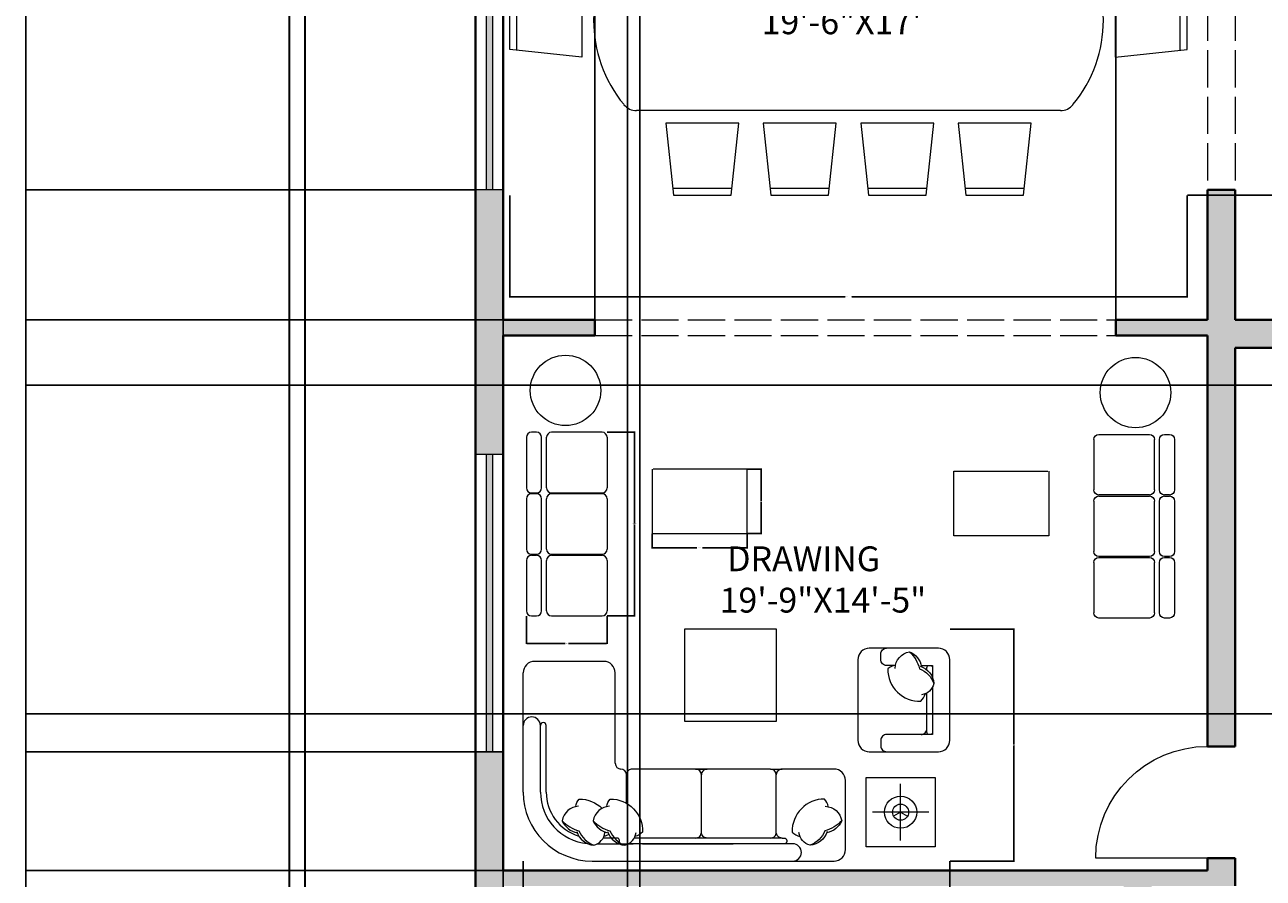
# Model space of a CAD drawing. Units: inches. Extents: x 2330 to 3943, y 1763 to 3461.
# Tile 10 of 40: x 2330 to 2730, y 2554 to 2829. Entities that reach past the tile are written whole.
import ezdxf

# ---------------------------------------------------------------- set-up
doc = ezdxf.new("R2010")
doc.units = ezdxf.units.IN
doc.linetypes.add('ACAD_ISO02W100', pattern=[15, 12, -3])
for name, color, linetype, lineweight in [('A-ANNO-DIMS', 2, 'Continuous', 18), ('A-AREA-IDEN', 7, 'Continuous', 18), ('A-DOOR', 4, 'Continuous', 18), ('A-FURN', 8, 'Continuous', 13), ('A-GLAZ', 4, 'Continuous', 18), ('A-WALL', 7, 'Continuous', 40), ('A-WALL-OVHD', 7, 'ACAD_ISO02W100', 18), ('A-WALL-PATT', 252, 'Continuous', 13), ('C-PROP', 7, 'Continuous', 30)]:
    doc.layers.add(name, color=color, linetype=linetype, lineweight=lineweight)
doc.styles.get("Standard").update_dxf_attribs({"font": 'arial.ttf'})
doc.dimstyles.get("Standard").update_dxf_attribs({"dimtxt": 0.18, "dimasz": 0.18, "dimexe": 0.18, "dimexo": 0.0625, "dimgap": 0.09, "dimtad": 0, "dimtih": 1, "dimtoh": 1, "dimdec": 4, "dimzin": 0, "dimdsep": 46, "dimtxsty": 'Standard', "dimcen": 0.09, "dimadec": 0, "dimazin": 0, "dimtfac": 1, "dimtdec": 4, "dimtofl": 0, "dimtmove": 0, "dimatfit": 3, "dimfxl": 1, "dimtolj": 1, "dimtzin": 0, "dimarcsym": 0})

# ---------------------------------------------------------------- blocks, each defined once
blk = doc.blocks.new('A$C714C64AF')
for p, q in [((3108, 2017, -5499), (1005, 2017, -5499)), ((908, 1917, -5499), (908, 1317, -5499)), ((1365, 1867, -5499), (2793, 1867, -5499)), ((3508, 1417, -5499), (3508, 839, -5499)), ((3558, 1417, -5499), (3558, 839, -5499)), ((3708, 1417, -5499), (3708, 839, -5499)), ((1008, 1217, -5499), (1458, 1217, -5499)), ((1558, 1217, -5499), (1458, 1217, -5499)), ((1558, 1217, -5499), (2760, 1217, -5499)), ((2209, 1217, -5499), (2109, 1217, -5499)), ((2908, 1167, -5499), (2908, 381, -5499)), ((3708, 839, -5499), (3708, 381, -5499)), ((3008, 281, -5499), (3608, 281, -5499))]:
    blk.add_line(p, q)
at = {"elevation": -5499}
for points in [[(128, 1892), (728, 1892), (728, 1292), (128, 1292)], [(2306, 800), (1506, 800), (1506, 0), (2306, 0)]]:
    blk.add_lwpolyline(points, close=True, dxfattribs=at)
for points in [[(428, 1837), (428, 1347)], [(1884, 1867), (2670, 1867)], [(1458, 1817), (2743, 1817)], [(2944, 1817), (3012, 1817)], [(428, 1592), (367, 1627)], [(428, 1592), (489, 1627)], [(183, 1592), (673, 1592)], [(428, 1592), (428, 1522)], [(2810, 1515), (2810, 1267)], [(248, 317), (150, 317), (150, 422)]]:
    blk.add_lwpolyline(points, dxfattribs=at)
for points in [[(940, 1667, -0.14773), (1086, 1753, -0.213343), (1215, 1879)], [(1066, 1760, -0.306663), (1215, 1879, -0.30633), (1312, 1770)], [(1456, 1817), (1438, 1817, -0.414214), (1418, 1837), (1418, 1847, -0.414214), (1438, 1867)], [(2670, 1867), (1884, 1867, 0.414214)], [(2974, 1760, 0.306663), (2825, 1879, 0.30633), (2727, 1770)], [(3068, 1867), (2753, 1867, 0.415492)], [(3100, 1667, 0.14773), (2954, 1753, 0.213343), (2825, 1879)], [(3013, 1867), (2891, 1867, 0.414214), (2871, 1847), (2871, 1837, 0.414214), (2891, 1817), (2963, 1817, 0.414214)], [(3243, 1760, 0.306663), (3094, 1879, 0.30633), (2997, 1770)], [(3369, 1667, 0.14773), (3223, 1753, 0.213343), (3094, 1879)], [(1083, 1541, -0.356772), (940, 1667, -0.249542), (1070, 1771)], [(1058, 1544, 0.165541), (1089, 1478, 0.425989), (1370, 1765, 0.121523), (1303, 1804)], [(1458, 1817, -0.414214), (1508, 1767)], [(1558, 1817, 0.414214), (1508, 1767), (1508, 1267, 0.432452)], [(1558, 1817, 0.414214), (1508, 1767)], [(2109, 1817, -0.414214), (2159, 1767)], [(2209, 1817, 0.414214), (2159, 1767), (2159, 1267, 0.432452)], [(2209, 1817, 0.414214), (2159, 1767)], [(2982, 1544, -0.165541), (2951, 1478, -0.425989), (2670, 1765, -0.121523), (2737, 1804)], [(2957, 1541, 0.356772), (3100, 1667, 0.249542), (2970, 1771)], [(2964, 1785, -0.071865), (3006, 1804)], [(3226, 1541, 0.356772), (3369, 1667, 0.249542), (3239, 1771)], [(3251, 1544, -0.165541), (3220, 1478, -0.200231), (3022, 1559)], [(150, 505), (150, 917), (550, 917, 0.414214), (600, 967), (600, 1017, 0.414214), (550, 1067)], [(150, 505), (150, 917), (550, 917, 0.414214), (600, 967), (600, 1017, 0.414214), (550, 1067)], [(150, 505), (150, 897, -0.414214), (170, 917), (180, 917, -0.414214), (200, 897), (200, 555, -0.729729)], [(250, 917, 0.414214), (200, 867)], [(257, 324, -0.306663), (138, 474, -0.30633), (246, 571)], [(473, 317, 0.165541), (539, 347, 0.425989), (252, 628, 0.121523), (213, 562)], [(350, 198, -0.14773), (264, 345, -0.213343), (138, 474)], [(150, 337), (150, 422, -0.414213)], [(200, 355), (200, 337, -0.414214), (180, 317), (170, 317, -0.414214), (150, 337)], [(476, 342, -0.356772), (350, 198, -0.249542), (246, 328)], [(473, 317), (550, 317, -0.414214), (600, 267), (600, 217, -0.414214), (550, 167)]]:
    blk.add_lwpolyline(points, format="xyb", dxfattribs=at)
blk.add_lwpolyline([(0, 267, 0.414214), (100, 167), (700, 167, 0.414214), (800, 267), (800, 967, 0.414214), (700, 1067), (100, 1067, 0.414214), (0, 967)], format="xyb", close=True, dxfattribs=at)
for radius in [140, 70]:
    blk.add_circle((428, 1592, -5499), radius)
for centre, radius, start, end in [((1008, 1917, -5499), 100, 90, 180), ((1365, 1942, -5499), 75, 90, 270), ((3108, 1417, -5499), 600, 0, 90), ((3108, 1417, -5499), 450, 0, 84.5853), ((3108, 1417, -5499), 400, 0, 72.9371), ((1008, 1317, -5499), 100, 180, 270), ((1458, 1267, -5499), 50, 270, 0), ((1458, 1267, -5499), 50, 270, 0), ((1558, 1267, -5499), 50, 180, 270), ((1558, 1267, -5499), 50, 180, 270), ((2109, 1267, -5499), 50, 270, 0), ((2109, 1267, -5499), 50, 270, 0), ((2209, 1267, -5499), 50, 180, 270), ((2209, 1267, -5499), 50, 180, 270), ((2760, 1267, -5499), 50, 270, 0), ((2760, 1267, -5499), 50, 270, 0), ((2860, 1267, -5499), 50, 180, 270), ((2860, 1267, -5499), 50, 180, 270), ((2858, 1167, -5499), 50, 0, 90), ((3533, 839, -5499), 25, 180, 0), ((3633, 839, -5499), 75, 180, 0), ((3008, 381, -5499), 100, 180, 270), ((3608, 381, -5499), 100, 270, 0)]:
    blk.add_arc(centre, radius, start, end)
blk = doc.blocks.new('A$C113D154D')
for p, q in [((0.96, 1.7118), (1.0076, 2.1547)), ((1.0076, 2.1547), (1.3624, 2.1547)), ((1.3624, 2.1547), (1.41, 1.7118)), ((1.56, 1.7118), (1.6076, 2.1547)), ((1.6076, 2.1547), (1.9624, 2.1547)), ((1.9624, 2.1547), (2.01, 1.7118)), ((2.16, 1.7118), (2.2076, 2.1547)), ((2.2076, 2.1547), (2.5624, 2.1547)), ((2.5624, 2.1547), (2.61, 1.7118)), ((2.76, 1.7118), (2.8076, 2.1547)), ((2.8076, 2.1547), (3.1624, 2.1547)), ((3.1624, 2.1547), (3.21, 1.7118)), ((1.003, 2.1119), (1.367, 2.1119)), ((1.603, 2.1119), (1.967, 2.1119)), ((2.203, 2.1119), (2.567, 2.1119)), ((2.803, 2.1119), (3.167, 2.1119)), ((1.41, 1.7118), (0.96, 1.7118)), ((2.01, 1.7118), (1.56, 1.7118)), ((2.61, 1.7118), (2.16, 1.7118)), ((3.21, 1.7118), (2.76, 1.7118)), ((0.7802, 1.6333), (3.3898, 1.6333)), ((0, 1.2523), (0.4429, 1.2999)), ((0.4429, 1.2999), (0.4429, 0.8499)), ((3.7271, 1.2999), (3.7271, 0.8499)), ((4.17, 1.2523), (3.7271, 1.2999)), ((0, 0.8975), (0, 1.2523)), ((0.0429, 0.8929), (0.0429, 1.2569)), ((4.1272, 0.8929), (4.1272, 1.2569)), ((4.17, 0.8975), (4.17, 1.2523)), ((0.4429, 0.8499), (0, 0.8975)), ((3.7271, 0.8499), (4.17, 0.8975)), ((3.3898, 0.5214), (0.7802, 0.5214)), ((1.41, 0.4429), (0.96, 0.4429)), ((0.96, 0.4429), (1.0076, 0)), ((1.3624, 0), (1.41, 0.4429)), ((2.01, 0.4429), (1.56, 0.4429)), ((1.56, 0.4429), (1.6076, 0)), ((1.9624, 0), (2.01, 0.4429)), ((2.61, 0.4429), (2.16, 0.4429)), ((2.16, 0.4429), (2.2076, 0)), ((2.5624, 0), (2.61, 0.4429)), ((3.21, 0.4429), (2.76, 0.4429)), ((2.76, 0.4429), (2.8076, 0)), ((3.1624, 0), (3.21, 0.4429)), ((1.003, 0.0429), (1.367, 0.0429)), ((1.0076, 0), (1.3624, 0)), ((1.603, 0.0429), (1.967, 0.0429)), ((1.6076, 0), (1.9624, 0)), ((2.203, 0.0429), (2.567, 0.0429)), ((2.2076, 0), (2.5624, 0)), ((2.803, 0.0429), (3.167, 0.0429)), ((2.8076, 0), (3.1624, 0))]:
    blk.add_line(p, q)
for centre, radius, start, end in [((0.7802, 1.5333), 0.1, 90, 140.39755), ((3.3898, 1.5333), 0.1, 39.60245, 90), ((1.3313, 1.0774), 0.8152, 140.39755, 219.60245), ((2.8387, 1.0774), 0.8152, 320.39755, 39.60245), ((0.7802, 0.6214), 0.1, 219.60245, 270), ((3.3898, 0.6214), 0.1, 270, 320.39755)]:
    blk.add_arc(centre, radius, start, end)
blk = doc.blocks.new('TABLE-RECTANGULAR')
for p, q in [((0, 20.81), (0, 0)), ((30.57, 20.81), (0.32, 20.81)), ((30.57, 0), (30.57, 20.81)), ((0, 0), (30.57, 0))]:
    blk.add_line(p, q)
blk = doc.blocks.new('SOFA-3-SEAT')
for p, q in [((0, 57.57), (0, 41.3)), ((3.25, 59.19), (1.63, 59.19)), ((4.88, 41.3), (4.88, 57.57)), ((6.5, 41.3), (6.5, 57.57)), ((24.39, 59.19), (8.13, 59.19)), ((26.02, 57.57), (26.02, 45.3)), ((26.02, 46.62), (26.02, 41.3)), ((0, 37.73), (0, 21.47)), ((1.63, 39.68), (3.25, 39.68)), ((3.25, 39.35), (1.63, 39.35)), ((4.88, 21.47), (4.88, 37.73)), ((6.5, 21.47), (6.5, 37.73)), ((8.13, 39.68), (24.39, 39.68)), ((24.39, 39.35), (8.13, 39.35)), ((26.02, 37.73), (26.02, 25.46)), ((26.02, 26.78), (26.02, 21.47)), ((0, 17.89), (0, 1.63)), ((1.63, 19.84), (3.25, 19.84)), ((3.25, 19.51), (1.63, 19.51)), ((4.88, 1.63), (4.88, 17.89)), ((6.5, 1.63), (6.5, 17.89)), ((8.13, 19.84), (24.39, 19.84)), ((24.39, 19.51), (8.13, 19.51)), ((26.02, 17.89), (26.02, 5.62)), ((26.02, 6.94), (26.02, 1.63)), ((1.63, 0), (3.25, 0)), ((8.13, 0), (24.39, 0))]:
    blk.add_line(p, q)
for centre, start, end in [((1.63, 57.57), 90, 180), ((3.25, 57.57), 0, 90), ((8.13, 57.57), 90, 180), ((24.39, 57.57), 0, 90), ((1.63, 41.3), 180, 270), ((1.63, 41.3), 180, 270), ((3.25, 41.3), 270, 0), ((3.25, 41.3), 270, 0), ((8.13, 41.3), 180, 270), ((8.13, 41.3), 180, 270), ((24.39, 41.3), 270, 0), ((1.63, 37.73), 90, 180), ((3.25, 37.73), 0, 90), ((8.13, 37.73), 90, 180), ((24.39, 37.73), 0, 90), ((1.63, 21.47), 180, 270), ((1.63, 21.47), 180, 270), ((3.25, 21.47), 270, 0), ((3.25, 21.47), 270, 0), ((8.13, 21.47), 180, 270), ((8.13, 21.47), 180, 270), ((24.39, 21.47), 270, 0), ((1.63, 17.89), 90, 180), ((3.25, 17.89), 0, 90), ((8.13, 17.89), 90, 180), ((24.39, 17.89), 0, 90), ((1.63, 1.63), 180, 270), ((1.63, 1.63), 180, 270), ((3.25, 1.63), 270, 0), ((3.25, 1.63), 270, 0), ((8.13, 1.63), 180, 270), ((8.13, 1.63), 180, 270), ((24.39, 1.63), 270, 0)]:
    blk.add_arc(centre, 1.63, start, end)
blk = doc.blocks.new('DOOR-SINGLE-36IN')
blk.add_line((0, 0), (-36, 0))
blk.add_arc((0, 0), 36, 180, 270)
blk = doc.blocks.new('WINDOW-96IN')
h = blk.add_hatch(color=256)
h.dxf.hatch_style = 1
h.paths.add_polyline_path([(5.5, 96), (3.5, 96), (3.5, 0), (5.5, 0)])
for p, q in [((0, 96), (9, 96)), ((3.5, 96), (3.5, 0)), ((5.5, 96), (5.5, 0)), ((0, 0), (9, 0))]:
    blk.add_line(p, q)
blk = doc.blocks.new('WINDOW-120IN')
h = blk.add_hatch(color=256)
h.dxf.hatch_style = 1
h.paths.add_polyline_path([(120, 5.5), (0, 5.5), (0, 3.5), (120, 3.5)])
for p, q in [((0, 9), (0, 0)), ((120, 9), (120, 0)), ((120, 5.5), (0, 5.5)), ((120, 3.5), (0, 3.5))]:
    blk.add_line(p, q)
blk = doc.blocks.new('*D43')
at = {"layer": 'A-ANNO-DIMS', "color": 0, "lineweight": -2, "transparency": 16777216}
for p, q in [((2532.68, 2664.7), (2532.68, 2659.99)), ((2563.25, 2664.7), (2563.25, 2659.99)), ((2532.86, 2660.17), (2547, 2660.17)), ((2563.07, 2660.17), (2548.93, 2660.17))]:
    blk.add_line(p, q, dxfattribs=at)
at = {"layer": 'A-ANNO-DIMS', "color": 0, "transparency": 16777216}
for points in [[(2532.86, 2660.2), (2532.86, 2660.14), (2532.68, 2660.17)], [(2563.07, 2660.2), (2563.07, 2660.14), (2563.25, 2660.17)]]:
    blk.add_solid(points, dxfattribs=at)
at = {"layer": 'Defpoints', "color": 0, "transparency": 16777216}
for p in [(2532.68, 2664.76), (2563.25, 2664.76), (2563.25, 2660.17)]:
    blk.add_point(p, dxfattribs=at)
at = {"layer": 'A-ANNO-DIMS', "color": 0, "transparency": 16777216, "insert": (2547.97, 2660.17), "char_height": 0.18, "attachment_point": 5}
blk.add_mtext('\\A1;TABLE 31 TYP.', dxfattribs=at)
blk = doc.blocks.new('*D44')
at = {"layer": 'A-ANNO-DIMS', "color": 0, "lineweight": -2, "transparency": 16777216}
for p, q in [((2563.31, 2685.57), (2568.02, 2685.57)), ((2567.84, 2685.39), (2567.84, 2675.35)), ((2567.84, 2664.94), (2567.84, 2674.98)), ((2563.31, 2664.76), (2568.02, 2664.76))]:
    blk.add_line(p, q, dxfattribs=at)
at = {"layer": 'A-ANNO-DIMS', "color": 0, "transparency": 16777216}
for points in [[(2567.81, 2685.39), (2567.87, 2685.39), (2567.84, 2685.57)], [(2567.81, 2664.94), (2567.87, 2664.94), (2567.84, 2664.76)]]:
    blk.add_solid(points, dxfattribs=at)
at = {"layer": 'Defpoints', "color": 0, "transparency": 16777216}
for p in [(2563.25, 2685.57), (2567.84, 2685.57), (2563.25, 2664.76)]:
    blk.add_point(p, dxfattribs=at)
at = {"layer": 'A-ANNO-DIMS', "color": 0, "transparency": 16777216, "insert": (2567.84, 2675.17), "char_height": 0.18, "attachment_point": 5}
blk.add_mtext('\\A1;21 TYP.', dxfattribs=at)
blk = doc.blocks.new('*D45')
at = {"layer": 'A-ANNO-DIMS', "color": 0, "lineweight": -2, "transparency": 16777216}
for p, q in [((2518.18, 2697.44), (2527.18, 2697.44)), ((2527, 2697.26), (2527, 2668.03)), ((2527, 2638.43), (2527, 2667.66)), ((2518.18, 2638.25), (2527.18, 2638.25))]:
    blk.add_line(p, q, dxfattribs=at)
at = {"layer": 'A-ANNO-DIMS', "color": 0, "transparency": 16777216}
for points in [[(2526.97, 2697.26), (2527.03, 2697.26), (2527, 2697.44)], [(2526.97, 2638.43), (2527.03, 2638.43), (2527, 2638.25)]]:
    blk.add_solid(points, dxfattribs=at)
at = {"layer": 'Defpoints', "color": 0, "transparency": 16777216}
for p in [(2518.12, 2697.44), (2527, 2697.44), (2518.12, 2638.25)]:
    blk.add_point(p, dxfattribs=at)
at = {"layer": 'A-ANNO-DIMS', "color": 0, "transparency": 16777216, "insert": (2527, 2667.85), "char_height": 0.18, "attachment_point": 5}
blk.add_mtext('\\A1;SOFA 59 TYP.', dxfattribs=at)
blk = doc.blocks.new('*D46')
at = {"layer": 'A-ANNO-DIMS', "color": 0, "lineweight": -2, "transparency": 16777216}
for p, q in [((2492.1, 2638.19), (2492.1, 2629.19)), ((2518.12, 2638.19), (2518.12, 2629.19)), ((2492.28, 2629.37), (2504.58, 2629.37)), ((2517.94, 2629.37), (2505.64, 2629.37))]:
    blk.add_line(p, q, dxfattribs=at)
at = {"layer": 'A-ANNO-DIMS', "color": 0, "transparency": 16777216}
for points in [[(2492.28, 2629.4), (2492.28, 2629.34), (2492.1, 2629.37)], [(2517.94, 2629.4), (2517.94, 2629.34), (2518.12, 2629.37)]]:
    blk.add_solid(points, dxfattribs=at)
at = {"layer": 'Defpoints', "color": 0, "transparency": 16777216}
for p in [(2492.1, 2638.25), (2518.12, 2638.25), (2518.12, 2629.37)]:
    blk.add_point(p, dxfattribs=at)
at = {"layer": 'A-ANNO-DIMS', "color": 0, "transparency": 16777216, "insert": (2505.11, 2629.37), "char_height": 0.18, "attachment_point": 5}
blk.add_mtext('\\A1;26 TYP.', dxfattribs=at)
blk = doc.blocks.new('*D49')
at = {"layer": 'A-ANNO-DIMS', "color": 0, "lineweight": -2, "transparency": 16777216}
for p, q in [((2491.06, 2559.13), (2491.06, 2538.38)), ((2628.63, 2559.13), (2628.63, 2538.38)), ((2491.24, 2538.56), (2558.6, 2538.56)), ((2628.45, 2538.56), (2561.09, 2538.56))]:
    blk.add_line(p, q, dxfattribs=at)
at = {"layer": 'A-ANNO-DIMS', "color": 0, "transparency": 16777216}
for points in [[(2491.24, 2538.59), (2491.24, 2538.53), (2491.06, 2538.56)], [(2628.45, 2538.59), (2628.45, 2538.53), (2628.63, 2538.56)]]:
    blk.add_solid(points, dxfattribs=at)
at = {"layer": 'Defpoints', "color": 0, "transparency": 16777216}
for p in [(2491.06, 2559.19), (2628.63, 2559.19), (2491.06, 2538.56)]:
    blk.add_point(p, dxfattribs=at)
at = {"layer": 'A-ANNO-DIMS', "color": 0, "transparency": 16777216, "insert": (2559.84, 2538.56), "char_height": 0.18, "attachment_point": 5}
blk.add_mtext('\\A1;CORNER SOFA 138', dxfattribs=at)
blk = doc.blocks.new('*D50')
at = {"layer": 'A-ANNO-DIMS', "color": 0, "lineweight": -2, "transparency": 16777216}
for p, q in [((2628.69, 2634.01), (2649.44, 2634.01)), ((2649.26, 2633.83), (2649.26, 2596.78)), ((2649.26, 2559.37), (2649.26, 2596.42)), ((2628.69, 2559.19), (2649.44, 2559.19))]:
    blk.add_line(p, q, dxfattribs=at)
at = {"layer": 'A-ANNO-DIMS', "color": 0, "transparency": 16777216}
for points in [[(2649.23, 2633.83), (2649.29, 2633.83), (2649.26, 2634.01)], [(2649.23, 2559.37), (2649.29, 2559.37), (2649.26, 2559.19)]]:
    blk.add_solid(points, dxfattribs=at)
at = {"layer": 'Defpoints', "color": 0, "transparency": 16777216}
for p in [(2628.63, 2634.01), (2628.63, 2559.19), (2649.26, 2559.19)]:
    blk.add_point(p, dxfattribs=at)
at = {"layer": 'A-ANNO-DIMS', "color": 0, "transparency": 16777216, "insert": (2649.26, 2596.6), "char_height": 0.18, "attachment_point": 5}
blk.add_mtext('\\A1;75', dxfattribs=at)
blk = doc.blocks.new('*D51')
at = {"layer": 'A-ANNO-DIMS', "color": 0, "lineweight": -2, "transparency": 16777216}
for p, q in [((2486.74, 2773.8), (2486.74, 2740.92)), ((2705.15, 2773.8), (2705.15, 2740.92)), ((2486.92, 2741.1), (2594.91, 2741.1)), ((2704.97, 2741.1), (2596.99, 2741.1))]:
    blk.add_line(p, q, dxfattribs=at)
at = {"layer": 'A-ANNO-DIMS', "color": 0, "transparency": 16777216}
for points in [[(2486.92, 2741.13), (2486.92, 2741.07), (2486.74, 2741.1)], [(2704.97, 2741.13), (2704.97, 2741.07), (2705.15, 2741.1)]]:
    blk.add_solid(points, dxfattribs=at)
at = {"layer": 'Defpoints', "color": 0, "transparency": 16777216}
for p in [(2486.74, 2773.87), (2705.15, 2773.87), (2705.15, 2741.1)]:
    blk.add_point(p, dxfattribs=at)
at = {"layer": 'A-ANNO-DIMS', "color": 0, "transparency": 16777216, "insert": (2595.95, 2741.1), "char_height": 0.18, "attachment_point": 5}
blk.add_mtext('\\A1;DINING SET 218', dxfattribs=at)
blk = doc.blocks.new('*D52')
at = {"layer": 'A-ANNO-DIMS', "color": 0, "lineweight": -2, "transparency": 16777216}
for p, q in [((2705.22, 2886.72), (2738.1, 2886.72)), ((2737.92, 2886.54), (2737.92, 2830.48)), ((2737.92, 2774.05), (2737.92, 2830.11)), ((2705.22, 2773.87), (2738.1, 2773.87))]:
    blk.add_line(p, q, dxfattribs=at)
at = {"layer": 'A-ANNO-DIMS', "color": 0, "transparency": 16777216}
for points in [[(2737.89, 2886.54), (2737.95, 2886.54), (2737.92, 2886.72)], [(2737.89, 2774.05), (2737.95, 2774.05), (2737.92, 2773.87)]]:
    blk.add_solid(points, dxfattribs=at)
at = {"layer": 'Defpoints', "color": 0, "transparency": 16777216}
for p in [(2705.15, 2886.72), (2737.92, 2886.72), (2705.15, 2773.87)]:
    blk.add_point(p, dxfattribs=at)
at = {"layer": 'A-ANNO-DIMS', "color": 0, "transparency": 16777216, "insert": (2737.92, 2830.3), "char_height": 0.18, "attachment_point": 5}
blk.add_mtext('\\A1;113', dxfattribs=at)
blk = doc.blocks.new('*D60')
at = {"layer": 'A-ANNO-DIMS', "color": 0, "lineweight": -2, "transparency": 16777216}
for p, q in [((2415.6, 3210.65), (2330.5, 3210.65)), ((2330.68, 3210.47), (2330.68, 2592.83)), ((2330.68, 1974.83), (2330.68, 2592.47)), ((2415.6, 1974.65), (2330.5, 1974.65))]:
    blk.add_line(p, q, dxfattribs=at)
at = {"layer": 'A-ANNO-DIMS', "color": 0, "transparency": 16777216}
for points in [[(2330.65, 3210.47), (2330.71, 3210.47), (2330.68, 3210.65)], [(2330.65, 1974.83), (2330.71, 1974.83), (2330.68, 1974.65)]]:
    blk.add_solid(points, dxfattribs=at)
at = {"layer": 'Defpoints', "color": 0, "transparency": 16777216}
for p in [(2330.68, 3210.65), (2415.66, 3210.65), (2415.66, 1974.65)]:
    blk.add_point(p, dxfattribs=at)
at = {"layer": 'A-ANNO-DIMS', "color": 0, "transparency": 16777216, "insert": (2330.68, 2592.65), "char_height": 0.18, "attachment_point": 5}
blk.add_mtext('\\A1;1236', dxfattribs=at)
blk = doc.blocks.new('*D62')
at = {"layer": 'A-ANNO-DIMS', "color": 0, "lineweight": -2, "transparency": 16777216}
for p, q in [((2475.6, 3162.65), (2330.5, 3162.65)), ((2330.68, 3162.47), (2330.68, 2687.58)), ((2330.68, 2212.33), (2330.68, 2687.22)), ((2475.6, 2212.15), (2330.5, 2212.15))]:
    blk.add_line(p, q, dxfattribs=at)
at = {"layer": 'A-ANNO-DIMS', "color": 0, "transparency": 16777216}
for points in [[(2330.65, 3162.47), (2330.71, 3162.47), (2330.68, 3162.65)], [(2330.65, 2212.33), (2330.71, 2212.33), (2330.68, 2212.15)]]:
    blk.add_solid(points, dxfattribs=at)
at = {"layer": 'Defpoints', "color": 0, "transparency": 16777216}
for p in [(2330.68, 3162.65), (2475.66, 3162.65), (2475.66, 2212.15)]:
    blk.add_point(p, dxfattribs=at)
at = {"layer": 'A-ANNO-DIMS', "color": 0, "transparency": 16777216, "insert": (2330.68, 2687.4), "char_height": 0.18, "attachment_point": 5}
blk.add_mtext('\\A1;950.5', dxfattribs=at)
blk = doc.blocks.new('*D71')
at = {"layer": 'A-ANNO-DIMS', "color": 0, "lineweight": -2, "transparency": 16777216}
for p, q in [((2732.6, 2712.65), (2330.5, 2712.65)), ((2330.68, 2712.47), (2330.68, 2659.83)), ((2330.68, 2606.83), (2330.68, 2659.47)), ((2732.6, 2606.65), (2330.5, 2606.65))]:
    blk.add_line(p, q, dxfattribs=at)
at = {"layer": 'A-ANNO-DIMS', "color": 0, "transparency": 16777216}
for points in [[(2330.65, 2712.47), (2330.71, 2712.47), (2330.68, 2712.65)], [(2330.65, 2606.83), (2330.71, 2606.83), (2330.68, 2606.65)]]:
    blk.add_solid(points, dxfattribs=at)
at = {"layer": 'Defpoints', "color": 0, "transparency": 16777216}
for p in [(2330.68, 2712.65), (2732.66, 2712.65), (2732.66, 2606.65)]:
    blk.add_point(p, dxfattribs=at)
at = {"layer": 'A-ANNO-DIMS', "color": 0, "transparency": 16777216, "insert": (2330.68, 2659.65), "char_height": 0.18, "attachment_point": 5}
blk.add_mtext('\\A1;106', dxfattribs=at)
blk = doc.blocks.new('*D79')
at = {"layer": 'A-ANNO-DIMS', "color": 0, "lineweight": -2, "transparency": 16777216}
for p, q in [((2484.66, 2221.21), (2484.66, 3461.3)), ((2484.84, 3461.12), (2504.44, 3461.12)), ((2524.48, 3461.12), (2504.88, 3461.12)), ((2524.66, 2221.21), (2524.66, 3461.3))]:
    blk.add_line(p, q, dxfattribs=at)
at = {"layer": 'A-ANNO-DIMS', "color": 0, "transparency": 16777216}
for points in [[(2484.84, 3461.15), (2484.84, 3461.09), (2484.66, 3461.12)], [(2524.48, 3461.15), (2524.48, 3461.09), (2524.66, 3461.12)]]:
    blk.add_solid(points, dxfattribs=at)
at = {"layer": 'Defpoints', "color": 0, "transparency": 16777216}
for p in [(2524.66, 3461.12), (2484.66, 2221.15), (2524.66, 2221.15)]:
    blk.add_point(p, dxfattribs=at)
at = {"layer": 'A-ANNO-DIMS', "color": 0, "transparency": 16777216, "insert": (2504.66, 3461.12), "char_height": 0.18, "attachment_point": 5}
blk.add_mtext('\\A1;40', dxfattribs=at)
blk = doc.blocks.new('*D81')
at = {"layer": 'A-ANNO-DIMS', "color": 0, "lineweight": -2, "transparency": 16777216}
for p, q in [((2484.6, 2594.4), (2330.5, 2594.4)), ((2330.68, 2594.22), (2330.68, 2575.46)), ((2330.68, 2556.33), (2330.68, 2575.1)), ((2484.6, 2556.15), (2330.5, 2556.15))]:
    blk.add_line(p, q, dxfattribs=at)
at = {"layer": 'A-ANNO-DIMS', "color": 0, "transparency": 16777216}
for points in [[(2330.65, 2594.22), (2330.71, 2594.22), (2330.68, 2594.4)], [(2330.65, 2556.33), (2330.71, 2556.33), (2330.68, 2556.15)]]:
    blk.add_solid(points, dxfattribs=at)
at = {"layer": 'Defpoints', "color": 0, "transparency": 16777216}
for p in [(2330.68, 2594.4), (2484.66, 2594.4), (2484.66, 2556.15)]:
    blk.add_point(p, dxfattribs=at)
at = {"layer": 'A-ANNO-DIMS', "color": 0, "transparency": 16777216, "insert": (2330.68, 2575.28), "char_height": 0.18, "attachment_point": 5}
blk.add_mtext('\\A1;38.25', dxfattribs=at)
blk = doc.blocks.new('*D82')
at = {"layer": 'A-ANNO-DIMS', "color": 0, "lineweight": -2, "transparency": 16777216}
for p, q in [((2475.6, 2775.65), (2330.5, 2775.65)), ((2330.68, 2775.47), (2330.68, 2754.83)), ((2330.68, 2733.83), (2330.68, 2754.47)), ((2484.6, 2733.65), (2330.5, 2733.65))]:
    blk.add_line(p, q, dxfattribs=at)
at = {"layer": 'A-ANNO-DIMS', "color": 0, "transparency": 16777216}
for points in [[(2330.65, 2775.47), (2330.71, 2775.47), (2330.68, 2775.65)], [(2330.65, 2733.83), (2330.71, 2733.83), (2330.68, 2733.65)]]:
    blk.add_solid(points, dxfattribs=at)
at = {"layer": 'Defpoints', "color": 0, "transparency": 16777216}
for p in [(2330.68, 2775.65), (2475.66, 2775.65), (2484.66, 2733.65)]:
    blk.add_point(p, dxfattribs=at)
at = {"layer": 'A-ANNO-DIMS', "color": 0, "transparency": 16777216, "insert": (2330.68, 2754.65), "char_height": 0.18, "attachment_point": 5}
blk.add_mtext('\\A1;42', dxfattribs=at)
blk = doc.blocks.new('*D83')
at = {"layer": 'A-ANNO-DIMS', "color": 0, "lineweight": -2, "transparency": 16777216}
for p, q in [((2514.16, 2733.71), (2514.16, 3461.3)), ((2514.34, 3461.12), (2597.88, 3461.12)), ((2681.98, 3461.12), (2598.44, 3461.12)), ((2682.16, 2733.71), (2682.16, 3461.3))]:
    blk.add_line(p, q, dxfattribs=at)
at = {"layer": 'A-ANNO-DIMS', "color": 0, "transparency": 16777216}
for points in [[(2514.34, 3461.15), (2514.34, 3461.09), (2514.16, 3461.12)], [(2681.98, 3461.15), (2681.98, 3461.09), (2682.16, 3461.12)]]:
    blk.add_solid(points, dxfattribs=at)
at = {"layer": 'Defpoints', "color": 0, "transparency": 16777216}
for p in [(2682.16, 3461.12), (2514.16, 2733.65), (2682.16, 2733.65)]:
    blk.add_point(p, dxfattribs=at)
at = {"layer": 'A-ANNO-DIMS', "color": 0, "transparency": 16777216, "insert": (2598.16, 3461.12), "char_height": 0.18, "attachment_point": 5}
blk.add_mtext('\\A1;168', dxfattribs=at)
blk = doc.blocks.new('*D84')
at = {"layer": 'A-ANNO-DIMS', "color": 0, "lineweight": -2, "transparency": 16777216}
for p, q in [((2484.66, 2733.71), (2484.66, 3461.3)), ((2484.84, 3461.12), (2499.08, 3461.12)), ((2513.98, 3461.12), (2499.74, 3461.12)), ((2514.16, 2733.71), (2514.16, 3461.3))]:
    blk.add_line(p, q, dxfattribs=at)
at = {"layer": 'A-ANNO-DIMS', "color": 0, "transparency": 16777216}
for points in [[(2484.84, 3461.15), (2484.84, 3461.09), (2484.66, 3461.12)], [(2513.98, 3461.15), (2513.98, 3461.09), (2514.16, 3461.12)]]:
    blk.add_solid(points, dxfattribs=at)
at = {"layer": 'Defpoints', "color": 0, "transparency": 16777216}
for p in [(2514.16, 3461.12), (2484.66, 2733.65), (2514.16, 2733.65)]:
    blk.add_point(p, dxfattribs=at)
at = {"layer": 'A-ANNO-DIMS', "color": 0, "transparency": 16777216, "insert": (2499.41, 3461.12), "char_height": 0.18, "attachment_point": 5}
blk.add_mtext('\\A1;29.5', dxfattribs=at)
blk = doc.blocks.new('*D90')
at = {"layer": 'A-ANNO-DIMS', "color": 0, "lineweight": -2, "transparency": 16777216}
for p, q in [((2484.66, 3153.59), (2484.66, 1901.2)), ((2528.66, 3153.59), (2528.66, 1901.2)), ((2484.84, 1901.38), (2506.44, 1901.38)), ((2528.48, 1901.38), (2506.88, 1901.38))]:
    blk.add_line(p, q, dxfattribs=at)
at = {"layer": 'A-ANNO-DIMS', "color": 0, "transparency": 16777216}
for points in [[(2484.84, 1901.41), (2484.84, 1901.35), (2484.66, 1901.38)], [(2528.48, 1901.41), (2528.48, 1901.35), (2528.66, 1901.38)]]:
    blk.add_solid(points, dxfattribs=at)
at = {"layer": 'Defpoints', "color": 0, "transparency": 16777216}
for p in [(2484.66, 3153.65), (2528.66, 3153.65), (2528.66, 1901.38)]:
    blk.add_point(p, dxfattribs=at)
at = {"layer": 'A-ANNO-DIMS', "color": 0, "transparency": 16777216, "insert": (2506.66, 1901.38), "char_height": 0.18, "attachment_point": 5}
blk.add_mtext('\\A1;44', dxfattribs=at)

msp = doc.modelspace()

# ---------------------------------------------------------------- hatches: boundary and pattern name
at = {"layer": 'A-WALL-PATT'}
h = msp.add_hatch(color=256, dxfattribs=at)
h.dxf.hatch_style = 1
h.paths.add_polyline_path([(2484.6605, 2775.6524), (2475.6605, 2775.6524), (2475.6605, 2690.4024), (2484.6605, 2690.4024), (2484.6605, 2728.6524), (2514.1605, 2728.6524), (2514.1605, 2733.6524), (2484.6605, 2733.6524)])
h = msp.add_hatch(color=256, dxfattribs=at)
h.dxf.hatch_style = 1
h.paths.add_polyline_path([(2920.6605, 2733.6524), (2720.6605, 2733.6524), (2720.6605, 2775.6524), (2711.6605, 2775.6524), (2711.6605, 2733.6524), (2682.1605, 2733.6524), (2682.1605, 2728.6524), (2711.6605, 2728.6524), (2711.6605, 2596.1524), (2720.6605, 2596.1524), (2720.6605, 2724.6524), (2920.6605, 2724.6524)])
h = msp.add_hatch(color=256, dxfattribs=at)
h.dxf.hatch_style = 1
h.paths.add_polyline_path([(2484.6605, 2594.4024), (2475.6605, 2594.4024), (2475.6605, 2523.7574), (2484.6605, 2523.7574), (2484.6605, 2551.1524), (2684.6605, 2551.1524), (2684.6605, 2547.1524), (2693.6605, 2547.1524), (2693.6605, 2551.1524), (2720.6605, 2551.1524), (2720.6605, 2560.1524), (2711.6605, 2560.1524), (2711.6605, 2556.1524), (2484.6605, 2556.1524)])

# ---------------------------------------------------------------- linework, layer by layer
at = {"layer": 'A-FURN'}
for centre in [(2504.7108, 2710.9405), (2688.4815, 2710.2324)]:
    msp.add_circle(centre, 11.3598, dxfattribs=at)
at = {"layer": 'A-WALL'}
for p, q in [((2475.6605, 3162.6524), (2475.6605, 2212.1524)), ((2484.6605, 2937.6524), (2484.6605, 2733.6524)), ((2711.6605, 2775.6524), (2720.6605, 2775.6524)), ((2711.6605, 2775.6524), (2711.6605, 2733.6524)), ((2720.6605, 2775.6524), (2720.6605, 2733.6524)), ((2484.6605, 2733.6524), (2514.1605, 2733.6524)), ((2514.1605, 2733.6524), (2514.1605, 2728.6524)), ((2682.1605, 2733.6524), (2682.1605, 2728.6524)), ((2682.1605, 2733.6524), (2711.6605, 2733.6524)), ((2720.6605, 2733.6524), (2920.6605, 2733.6524)), ((2484.6605, 2728.6524), (2514.1605, 2728.6524)), ((2484.6605, 2728.6524), (2484.6605, 2556.1524)), ((2682.1605, 2728.6524), (2711.6605, 2728.6524)), ((2711.6605, 2728.6524), (2711.6605, 2596.1524)), ((2720.6605, 2724.6524), (2920.6605, 2724.6524)), ((2720.6605, 2724.6524), (2720.6605, 2596.1524)), ((2711.6605, 2596.1524), (2720.6605, 2596.1524)), ((2711.6605, 2560.1524), (2720.6605, 2560.1524)), ((2711.6605, 2560.1524), (2711.6605, 2556.1524)), ((2720.6605, 2560.1524), (2720.6605, 2551.1524)), ((2484.6605, 2556.1524), (2711.6605, 2556.1524))]:
    msp.add_line(p, q, dxfattribs=at)
at = {"layer": 'A-WALL-OVHD'}
for p, q in [((2711.6605, 2895.6524), (2711.6605, 2775.6524)), ((2720.6605, 2895.6524), (2720.6605, 2775.6524)), ((2514.1605, 2733.6524), (2682.1605, 2733.6524)), ((2514.1605, 2728.6524), (2682.1605, 2728.6524))]:
    msp.add_line(p, q, dxfattribs=at)
at = {"layer": 'C-PROP'}
for p, q in [((2415.6605, 3210.6524), (2415.6605, 1974.6524)), ((2420.6605, 3205.6524), (2420.6605, 1979.6524))]:
    msp.add_line(p, q, dxfattribs=at)

# ---------------------------------------------------------------- block references
at = {"layer": 'A-DOOR', "extrusion": (0, 0, -1), "zscale": -1, "rotation": 180}
msp.add_blockref('DOOR-SINGLE-36IN', (-2711.6605, 2560.1524), dxfattribs=at)
at = {"layer": 'A-FURN', "xscale": 52.37726238140837, "yscale": 52.37726238140837, "zscale": 52.37726238140837}
msp.add_blockref('A$C113D154D', (2486.7408, 2773.8664), dxfattribs=at)
at = {"layer": 'A-FURN'}
for name, p in [('SOFA-3-SEAT', (2492.1027, 2638.2516)), ('TABLE-RECTANGULAR', (2532.681, 2664.758))]:
    msp.add_blockref(name, p, dxfattribs=at)
at = {"layer": 'A-FURN', "extrusion": (0, 0, -1), "zscale": -1}
for name, p in [('SOFA-3-SEAT', (-2701.0896, 2637.5435)), ('TABLE-RECTANGULAR', (-2660.5113, 2664.0499))]:
    msp.add_blockref(name, p, dxfattribs=at)
at = {"layer": 'A-FURN', "xscale": 0.0370987246016696, "yscale": 0.0370987246016696, "zscale": 0.0370987246016696, "rotation": 180}
msp.add_blockref('A$C714C64AF', (2628.6266, 2634.0128), dxfattribs=at)
at = {"layer": 'A-GLAZ', "extrusion": (0, 0, -1), "zscale": -1, "rotation": 90.00000000000006}
msp.add_blockref('WINDOW-120IN', (-2475.6605, 2775.6524), dxfattribs=at)
at = {"layer": 'A-GLAZ'}
msp.add_blockref('WINDOW-96IN', (2475.6605, 2594.4024), dxfattribs=at)

# ---------------------------------------------------------------- texts
at = {"layer": 'A-AREA-IDEN', "char_height": 8, "attachment_point": 1}
for s, width, insert in [(' DINING\\P19\'-6"X17\'', 93.76933, (2567.9313, 2847.1316)), (' DRAWING\\P19\'-9"X14\'-5"', 124.077959, (2554.4262, 2660.6441))]:
    msp.add_mtext_dynamic_manual_height_columns(s, width=width, gutter_width=12.5, heights=[0], dxfattribs=dict(at, insert=insert))

# ---------------------------------------------------------------- dimensions: what is measured, and where the dimension line sits
at = {"layer": 'A-ANNO-DIMS'}
for base, p1, p2, override, picture, middle in [((2524.6605, 3461.1231), (2484.6605, 2221.1524), (2524.6605, 2221.1524), {"dimdec": 0, "dimlfac": 1, "dimrnd": 0, "dimzin": 0, "dimdsep": 46, "dimlunit": 2}, '*D79', (2504.6605, 3461.1231)), ((2514.1605, 3461.1231), (2484.6605, 2733.6524), (2514.1605, 2733.6524), {"dimdec": 1, "dimlfac": 1, "dimrnd": 0, "dimzin": 0, "dimdsep": 46, "dimlunit": 2}, '*D84', (2499.4105, 3461.1231)), ((2682.1605, 3461.1231), (2514.1605, 2733.6524), (2682.1605, 2733.6524), {"dimdec": 0, "dimlfac": 1, "dimrnd": 0, "dimzin": 0, "dimdsep": 46, "dimlunit": 2}, '*D83', (2598.1605, 3461.1231)), ((2528.6605, 1901.3774), (2484.6605, 3153.6524), (2528.6605, 3153.6524), {"dimdec": 0, "dimlfac": 1, "dimrnd": 0, "dimzin": 0, "dimdsep": 46, "dimlunit": 2}, '*D90', (2506.6605, 1901.3774))]:
    dim = msp.add_linear_dim(base=base, p1=p1, p2=p2, dimstyle='Standard', override=override, dxfattribs=at)
    dim.commit()
    dim.dimension.update_dxf_attribs({"geometry": picture, "text_midpoint": middle})
for base, p1, p2, angle, override, picture, middle in [((2330.6824, 3210.6524), (2415.6605, 1974.6524), (2415.6605, 3210.6524), 90, {"dimdec": 0, "dimlfac": 1, "dimrnd": 0, "dimzin": 0, "dimdsep": 46, "dimlunit": 2}, '*D60', (2330.6824, 2592.6524)), ((2330.6824, 3162.6524), (2475.6605, 2212.1524), (2475.6605, 3162.6524), 90, {"dimdec": 1, "dimlfac": 1, "dimrnd": 0, "dimzin": 0, "dimdsep": 46, "dimlunit": 2}, '*D62', (2330.6824, 2687.4024)), ((2737.9166, 2886.7243), (2705.1545, 2773.8664), (2705.1545, 2886.7243), 90, {"dimdec": 0, "dimlfac": 1, "dimrnd": 0, "dimzin": 0, "dimdsep": 46, "dimlunit": 2}, '*D52', (2737.9166, 2830.2954)), ((2330.6824, 2775.6524), (2484.6605, 2733.6524), (2475.6605, 2775.6524), 90, {"dimdec": 0, "dimlfac": 1, "dimrnd": 0, "dimzin": 0, "dimdsep": 46, "dimlunit": 2}, '*D82', (2330.6824, 2754.6524)), ((2330.6824, 2712.6524), (2732.6605, 2606.6524), (2732.6605, 2712.6524), 90, {"dimdec": 0, "dimlfac": 1, "dimrnd": 0, "dimzin": 0, "dimdsep": 46, "dimlunit": 2}, '*D71', (2330.6824, 2659.6524)), ((2649.2614, 2559.1906), (2628.6266, 2634.0128), (2628.6266, 2559.1906), 270, {"dimdec": 0, "dimlfac": 1, "dimrnd": 0, "dimzin": 0, "dimdsep": 46, "dimlunit": 2}, '*D50', (2649.2614, 2596.6017)), ((2330.6824, 2594.4024), (2484.6605, 2556.1524), (2484.6605, 2594.4024), 90, {"dimdec": 2, "dimlfac": 1, "dimrnd": 0, "dimzin": 0, "dimdsep": 46, "dimlunit": 2}, '*D81', (2330.6824, 2575.2774))]:
    dim = msp.add_linear_dim(base=base, p1=p1, p2=p2, angle=angle, dimstyle='Standard', override=override, dxfattribs=at)
    dim.commit()
    dim.dimension.update_dxf_attribs({"geometry": picture, "text_midpoint": middle})
for base, p1, p2, text, picture, middle in [((2705.1545, 2741.1044), (2486.7408, 2773.8664), (2705.1545, 2773.8664), 'DINING SET <>', '*D51', (2595.9477, 2741.1044)), ((2563.2522, 2660.1721), (2532.6806, 2664.7579), (2563.2522, 2664.7579), 'TABLE <> TYP.', '*D43', (2547.9664, 2660.1721)), ((2518.1211, 2629.3728), (2492.1027, 2638.2516), (2518.1211, 2638.2516), '<> TYP.', '*D46', (2505.1119, 2629.3728))]:
    dim = msp.add_linear_dim(base=base, p1=p1, p2=p2, text=text, dimstyle='Standard', override={"dimdec": 0, "dimlfac": 1, "dimrnd": 0, "dimzin": 0, "dimdsep": 46, "dimlunit": 2}, dxfattribs=at)
    dim.commit()
    dim.dimension.update_dxf_attribs({"geometry": picture, "text_midpoint": middle})
for base, p1, p2, angle, text, picture, middle in [((2526.9999, 2697.4435), (2518.1211, 2638.2516), (2518.1211, 2697.4435), 90, 'SOFA <> TYP.', '*D45', (2526.9999, 2667.8475)), ((2567.838, 2685.5726), (2563.2522, 2664.7579), (2563.2522, 2685.5726), 90, '<> TYP.', '*D44', (2567.838, 2675.1652)), ((2491.0616, 2538.5559), (2628.6266, 2559.1906), (2491.0616, 2559.1906), 180, 'CORNER SOFA <>', '*D49', (2559.8441, 2538.5559))]:
    dim = msp.add_linear_dim(base=base, p1=p1, p2=p2, angle=angle, text=text, dimstyle='Standard', override={"dimdec": 0, "dimlfac": 1, "dimrnd": 0, "dimzin": 0, "dimdsep": 46, "dimlunit": 2}, dxfattribs=at)
    dim.commit()
    dim.dimension.update_dxf_attribs({"geometry": picture, "text_midpoint": middle})

doc.saveas('drawing.dxf')
